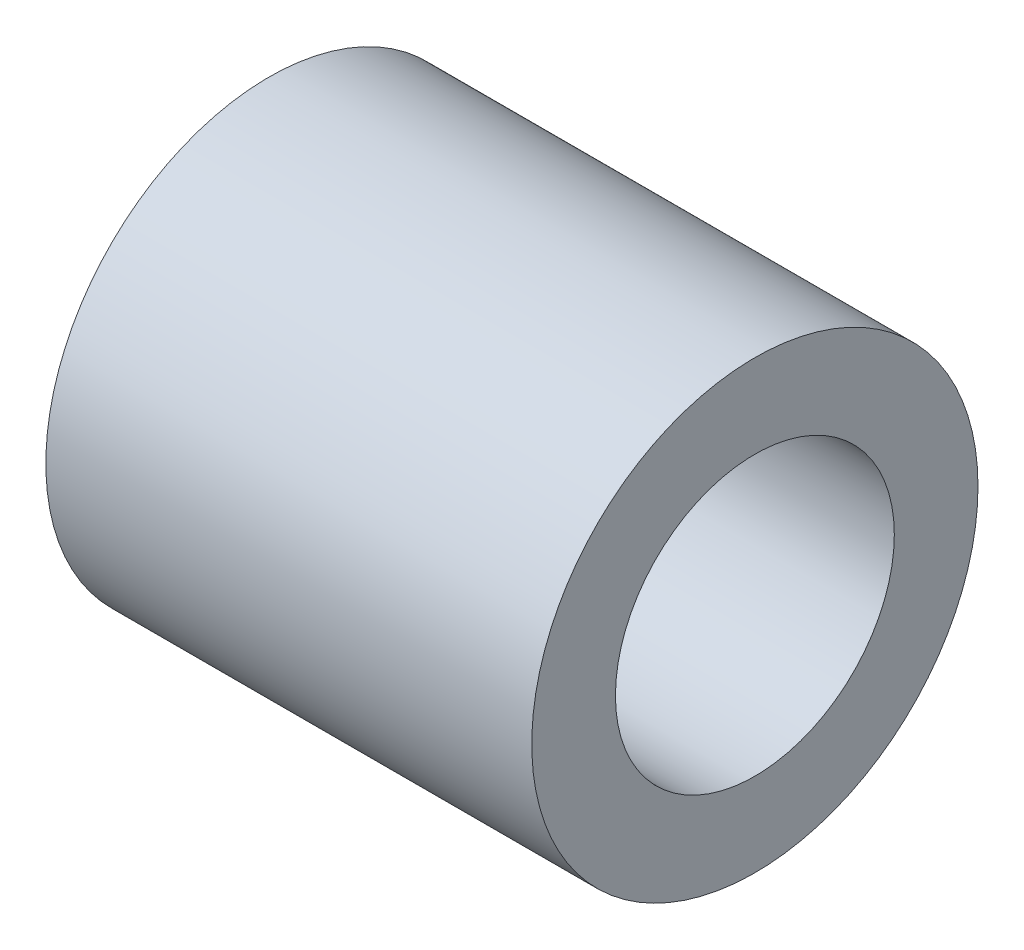
from build123d import *

# Parameters (mm, degrees)
CAP_BODY_SKETCH_8_R = 4
CAP_BODY_8X9_DEPTH  = 9
BORE_SKETCH_5_R     = 2.5
BORE_5X6_DEPTH      = 6


with BuildPart() as part:
    # Cap Body Sketch Ø8 → Cap Body Ø8x9 (new body)
    with BuildSketch(Plane(origin=(0, 0, 0), x_dir=(0, 0, -1), z_dir=(1, 0, 0))):
        Circle(CAP_BODY_SKETCH_8_R)
    extrude(amount=CAP_BODY_8X9_DEPTH)

    # Bore Drill Point Sketch → Bore Drill Point Cut (revolve, cut)
    with BuildSketch(Plane.XY, mode=Mode.PRIVATE) as bore_drill_point_cut_sk:
        Polygon((0, 3.5), (0.700208968, 4.712797508), (0, 4.712797508), align=None)
    revolve(bore_drill_point_cut_sk.sketch.rotate(Axis((-1000, 0, 0), (1, 0, 0)), 270), axis=Axis((-1000, 0, 0), (1, 0, 0)), mode=Mode.SUBTRACT)

    # Bore Sketch Ø5 → Bore Ø5x6 (cut)
    with BuildSketch(Plane(origin=(9, 0, 0), x_dir=(0, 0, -1), z_dir=(1, 0, 0))):
        Circle(BORE_SKETCH_5_R)
    extrude(amount=-BORE_5X6_DEPTH, mode=Mode.SUBTRACT)


solid = part.part
